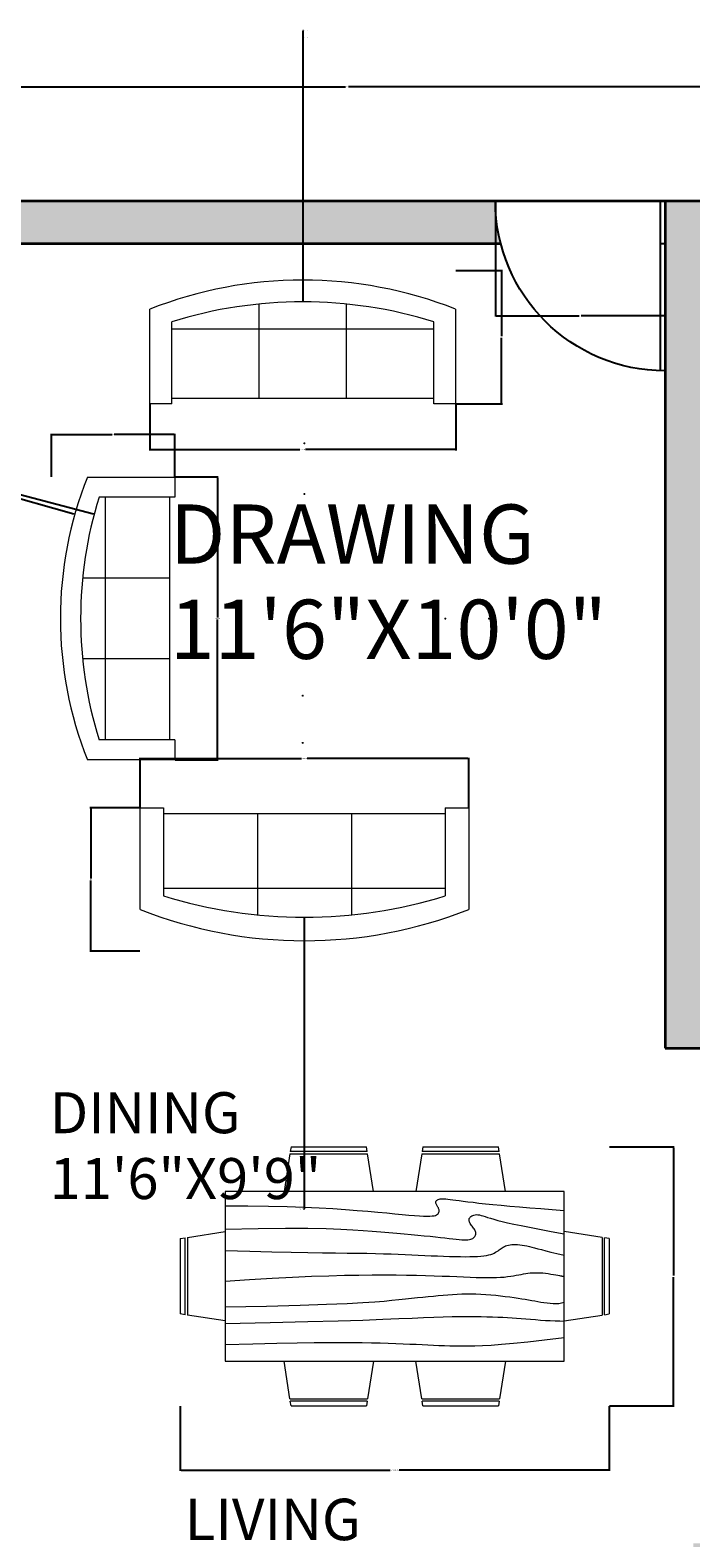
# Model space of a CAD drawing. Units: inches. Extents: x 582 to 1090, y 270 to 781.
# Tile 4 of 5: x 769 to 909, y 461 to 781. Entities that reach past the tile are written whole.
import ezdxf

# ---------------------------------------------------------------- set-up
doc = ezdxf.new("R2010")
doc.units = ezdxf.units.IN
doc.header["$MEASUREMENT"] = 0
for name, color, linetype, lineweight in [('A-ANNO-DIMS', 2, 'Continuous', 18), ('A-AREA-IDEN', 7, 'Continuous', 25), ('A-DOOR', 3, 'Continuous', 25), ('A-FURN', 8, 'Continuous', 18), ('A-WALL', 7, 'Continuous', 35)]:
    doc.layers.add(name, color=color, linetype=linetype, lineweight=lineweight)
doc.layers.add('A-WALL-PATT', color=9, linetype='Continuous', lineweight=13, true_color=0xc7c8ca)
doc.styles.get("Standard").update_dxf_attribs({"font": 'arial.ttf'})
doc.dimstyles.get("Standard").update_dxf_attribs({"dimtxt": 0.18, "dimasz": 0.18, "dimexe": 0.18, "dimexo": 0.0625, "dimgap": 0.09, "dimtad": 0, "dimtih": 1, "dimtoh": 1, "dimdec": 0, "dimzin": 0, "dimdsep": 46, "dimlunit": 3, "dimtxsty": 'Standard', "dimcen": 0.09, "dimadec": 0, "dimazin": 0, "dimtfac": 1, "dimtdec": 0, "dimtofl": 0, "dimtmove": 0, "dimatfit": 3, "dimfxl": 1, "dimtolj": 1, "dimtzin": 0, "dimarcsym": 0})

# ---------------------------------------------------------------- blocks, each defined once
blk = doc.blocks.new('Sofa - Roundback 7 ft.')
for p, q in [((-12.00002, -32.4421), (-12.00003, -6.5971)), ((11.99997, -32.4421), (11.99998, -6.5971)), ((-36.000027, -34), (-36.000027, -11.4696)), ((35.99998, -34), (35.99998, -11.4696)), ((-35.999844, -13.3819), (35.9998, -13.3819)), ((-36.000027, -32.4421), (35.99998, -32.4421))]:
    blk.add_line(p, q)
for points in [[(-36.000027, -34), (-42.000027, -34), (-42.000027, -8)], [(41.99998, -8), (41.99998, -34), (35.99998, -34)]]:
    blk.add_lwpolyline(points)
for centre, radius, start, end in [((0, -114.25), 114.25, 68.43141, 111.5686), ((-0.00001, -127.1968), 121.1968, 72.72033, 107.2797)]:
    blk.add_arc(centre, radius, start, end)
blk = doc.blocks.new('Dining Set - 36 x 72 in.')
for p, q in [((-22.2343, 26.00059), (-23.4847, 17.99762)), ((-22.2304, 26), (-5.7608, 26)), ((-22, 27.5), (-22.1562, 26.50042)), ((-5.8416, 26.5), (-22.1534, 26.5)), ((-22, 27.5), (-6, 27.5)), ((-5.8437, 26.49966), (-6, 27.5)), ((-4.5152, 17.99762), (-5.7655, 25.99926)), ((5.7657, 26.00059), (4.5153, 17.99762)), ((5.7696, 26), (22.2392, 26)), ((6, 27.5), (5.8438, 26.50042)), ((22.1584, 26.5), (5.8466, 26.5)), ((6, 27.5), (22, 27.5)), ((22.1563, 26.49966), (22, 27.5)), ((23.4848, 17.99762), (22.2345, 25.99926)), ((36, 18), (-36, 18)), ((-36, 18), (-36, -18)), ((36, -18), (36, 18)), ((-45.5, 8), (-44.5004, 8.15617)), ((-45.5, 8), (-45.5, -8)), ((-44.5, -8.15843), (-44.5, 8.15338)), ((-44.0006, 8.23428), (-35.9976, 9.48474)), ((-44, 8.23041), (-44, -8.23915)), ((44.0006, 8.23428), (35.9976, 9.48474)), ((44, 8.23041), (44, -8.23915)), ((44.5, -8.15843), (44.5, 8.15338)), ((45.5, 8), (44.5005, 8.15617)), ((45.5, 8), (45.5, -8)), ((-44.4997, -8.15631), (-45.5, -8)), ((-35.9976, -9.48476), (-43.9993, -8.2345)), ((35.9976, -9.48476), (43.9993, -8.2345)), ((44.4997, -8.15631), (45.5, -8)), ((-36, -18), (36, -18)), ((-22.2343, -26.0006), (-23.4847, -17.99762)), ((-4.5152, -17.99762), (-5.7655, -25.99928)), ((5.7657, -26.0006), (4.5153, -17.99762)), ((23.4848, -17.99762), (22.2345, -25.99928)), ((-22.2304, -26), (-5.7608, -26)), ((-22, -27.5), (-22.1562, -26.50044)), ((-5.8416, -26.5), (-22.1534, -26.5)), ((-22, -27.5), (-6, -27.5)), ((-5.8437, -26.49967), (-6, -27.5)), ((5.7696, -26), (22.2392, -26)), ((6, -27.5), (5.8438, -26.50044)), ((22.1584, -26.5), (5.8466, -26.5)), ((6, -27.5), (22, -27.5)), ((22.1563, -26.49967), (22, -27.5))]:
    blk.add_line(p, q)
for points in [[(-36, 15), (-31.1772, 14.97754), (-26.8079, 14.91406), (-22.8538, 14.81543), (-19.276, 14.6875), (-16.0362, 14.53613), (-13.0957, 14.36718), (-10.4159, 14.18652), (-7.9583, 14), (-5.6904, 13.81315), (-3.6035, 13.63021), (-1.6954, 13.45508), (0.0365, 13.29166), (1.5945, 13.14388), (2.9811, 13.01562), (4.1988, 12.9108), (5.25, 12.83333), (6.1393, 12.78613), (6.8802, 12.76823), (7.4883, 12.77767), (7.9792, 12.8125), (8.3685, 12.87077), (8.6719, 12.95052), (8.9049, 13.0498), (9.0833, 13.16666), (9.2205, 13.29899), (9.3216, 13.44401), (9.3895, 13.59879), (9.4271, 13.76041), (9.4373, 13.92594), (9.4232, 14.09245), (9.3875, 14.257), (9.3333, 14.41666), (9.2638, 14.56917), (9.1836, 14.71484), (9.0975, 14.85465), (9.0104, 14.98958), (8.9272, 15.1206), (8.8529, 15.2487), (8.7922, 15.37483), (8.75, 15.5), (8.7305, 15.62467), (8.7344, 15.74739), (8.7617, 15.86621), (8.8125, 15.97916), (8.8867, 16.08431), (8.9844, 16.17968), (9.1055, 16.26334), (9.25, 16.33333), (9.4189, 16.38802), (9.6172, 16.42708), (9.8506, 16.45052), (10.125, 16.45833), (10.4463, 16.45052), (10.8203, 16.42708), (11.2529, 16.38802), (11.75, 16.33333), (12.3184, 16.26318), (12.9694, 16.17838), (13.7151, 16.07991), (14.5677, 15.96875), (15.5395, 15.84586), (16.6426, 15.71224), (17.8893, 15.56884), (19.2917, 15.41666), (20.859, 15.25667), (22.5879, 15.08984), (24.4721, 14.91715), (26.5052, 14.73958), (28.6809, 14.5581), (30.9929, 14.3737), (33.4347, 14.18733), (36, 14)], [(-36, 10), (-28.9766, 10.14274), (-23.1725, 10.20442), (-18.4241, 10.19775), (-14.5677, 10.13541), (-11.4399, 10.03011), (-8.877, 9.89453), (-6.7154, 9.74137), (-4.7917, 9.58333), (-2.9698, 9.43082), (-1.2246, 9.28515), (0.4415, 9.14534), (2.026, 9.01041), (3.5266, 8.87939), (4.9408, 8.7513), (6.266, 8.62516), (7.5, 8.5), (8.6411, 8.37549), (9.6914, 8.2539), (10.6538, 8.13818), (11.5312, 8.03125), (12.3267, 7.93603), (13.043, 7.85547), (13.6831, 7.79248), (14.25, 7.75), (14.7471, 7.7303), (15.1797, 7.73307), (15.5537, 7.75732), (15.875, 7.80208), (16.1494, 7.86637), (16.3828, 7.94922), (16.5811, 8.04964), (16.75, 8.16666), (16.8944, 8.29915), (17.0143, 8.44531), (17.1089, 8.60319), (17.1771, 8.77083), (17.218, 8.94629), (17.2305, 9.1276), (17.2137, 9.31282), (17.1667, 9.5), (17.0895, 9.6875), (16.987, 9.875), (16.8649, 10.0625), (16.7292, 10.25), (16.5856, 10.4375), (16.4401, 10.625), (16.2985, 10.8125), (16.1667, 11), (16.05, 11.18733), (15.9518, 11.3737), (15.8752, 11.5581), (15.8229, 11.73958), (15.798, 11.91715), (15.8034, 12.08984), (15.842, 12.25667), (15.9167, 12.41666), (16.0295, 12.56836), (16.1784, 12.70833), (16.3605, 12.83268), (16.5729, 12.9375), (16.8127, 13.01888), (17.0768, 13.07291), (17.3625, 13.0957), (17.6667, 13.08333), (17.9894, 13.03312), (18.3418, 12.94726), (18.7382, 12.82918), (19.1927, 12.68229), (19.7195, 12.51001), (20.3327, 12.31575), (21.0465, 12.10294), (21.875, 11.875), (22.8357, 11.63354), (23.959, 11.37304), (25.2786, 11.08618), (26.8282, 10.76562), (28.6414, 10.40405), (30.752, 9.99414), (33.1936, 9.52856), (36, 9)], [(-36, 5.5), (-30.7157, 5.3348), (-26.069, 5.20963), (-21.9946, 5.11767), (-18.4271, 5.05208), (-15.3009, 5.00602), (-12.5508, 4.97265), (-10.1112, 4.94515), (-7.9167, 4.91666), (-5.909, 4.88167), (-4.0586, 4.83984), (-2.3429, 4.79215), (-0.7396, 4.73958), (0.7739, 4.6831), (2.22, 4.6237), (3.6213, 4.56233), (5, 4.5), (6.373, 4.43782), (7.7344, 4.3776), (9.0723, 4.32129), (10.375, 4.27083), (11.6309, 4.22819), (12.8281, 4.19531), (13.9551, 4.17415), (15, 4.16666), (15.954, 4.17448), (16.819, 4.19791), (17.6001, 4.23698), (18.3021, 4.29166), (18.9299, 4.36198), (19.4883, 4.44791), (19.9823, 4.54948), (20.4167, 4.66666), (20.7969, 4.79899), (21.1302, 4.94401), (21.4245, 5.09879), (21.6875, 5.26041), (21.9271, 5.42594), (22.1511, 5.59245), (22.3672, 5.757), (22.5834, 5.91666), (22.8065, 6.06868), (23.0404, 6.21093), (23.2879, 6.34147), (23.5521, 6.45833), (23.8358, 6.55957), (24.142, 6.64323), (24.4735, 6.70735), (24.8334, 6.75), (25.2235, 6.76969), (25.642, 6.76692), (26.0858, 6.74267), (26.5521, 6.69791), (27.0379, 6.63362), (27.5404, 6.55078), (28.0565, 6.45036), (28.5834, 6.33333), (29.1242, 6.19987), (29.7071, 6.04687), (30.3661, 5.87044), (31.1354, 5.66666), (32.0493, 5.43164), (33.142, 5.16146), (34.4475, 4.85221), (36, 4.5)], [(-36, -1), (-30.7915, -0.6591), (-26.0195, -0.38216), (-21.6519, -0.16284), (-17.6563, 0.00521), (-14.0005, 0.12833), (-10.6523, 0.21289), (-7.5796, 0.26522), (-4.75, 0.29166), (-2.134, 0.29793), (0.2878, 0.28711), (2.5317, 0.26163), (4.6146, 0.22396), (6.5529, 0.17651), (8.3633, 0.12174), (10.0623, 0.06209), (11.6667, 0), (13.1899, -0.06201), (14.6341, -0.1211), (15.9982, -0.17432), (17.2813, -0.21875), (18.4823, -0.25147), (19.6003, -0.26953), (20.6343, -0.27002), (21.5834, -0.25), (22.4481, -0.20768), (23.2357, -0.14584), (23.9549, -0.06836), (24.6146, 0.02083), (25.2235, 0.11784), (25.7904, 0.21875), (26.3241, 0.31966), (26.8334, 0.41666), (27.3265, 0.50618), (27.8099, 0.58593), (28.2894, 0.65397), (28.7709, 0.70833), (29.2601, 0.74707), (29.763, 0.76823), (30.2855, 0.76985), (30.8334, 0.75), (31.4088, 0.70784), (31.9994, 0.64713), (32.589, 0.57275), (33.1615, 0.48958), (33.7008, 0.4025), (34.1908, 0.3164), (34.6153, 0.23616), (34.9584, 0.16666), (35.2099, 0.11165), (35.3848, 0.07031), (35.504, 0.04069), (35.5886, 0.02083), (35.6594, 0.00879), (35.7377, 0.0026), (35.8442, 0.00032), (36, 0)], [(-36, -6.5), (-27.1843, -6.31267), (-20.084, -6.1263), (-14.469, -5.9419), (-10.1094, -5.76042), (-6.7752, -5.58285), (-4.2363, -5.41016), (-2.2629, -5.24333), (-0.625, -5.08334), (0.8708, -4.93099), (2.2715, -4.78646), (3.5872, -4.64974), (4.8281, -4.52084), (6.0046, -4.39974), (7.127, -4.28646), (8.2053, -4.18099), (9.25, -4.08334), (10.2705, -3.99382), (11.2734, -3.91407), (12.2647, -3.84603), (13.25, -3.79167), (14.2354, -3.75293), (15.2266, -3.73177), (16.2295, -3.73015), (17.25, -3.75), (18.2912, -3.79248), (19.3451, -3.85547), (20.4009, -3.93604), (21.4479, -4.03125), (22.4754, -4.13819), (23.4727, -4.25391), (24.4289, -4.37549), (25.3334, -4.5), (26.1785, -4.62492), (26.9694, -4.74935), (27.7145, -4.87281), (28.4219, -4.99479), (29.1, -5.11483), (29.7572, -5.23242), (30.4016, -5.34709), (31.0417, -5.45834), (31.6837, -5.56437), (32.3262, -5.65821), (32.9658, -5.73153), (33.599, -5.77604), (34.2224, -5.78345), (34.8327, -5.74545), (35.4264, -5.65373), (36, -5.5)], [(-36, -10), (-26.4022, -9.81299), (-18.4675, -9.62891), (-11.9839, -9.45069), (-6.7396, -9.28125), (-2.5226, -9.12354), (0.8789, -8.98047), (3.6769, -8.85498), (6.0833, -8.75), (8.2767, -8.66765), (10.3021, -8.60677), (12.1712, -8.56543), (13.8958, -8.54167), (15.4876, -8.53353), (16.9583, -8.53907), (18.3197, -8.55632), (19.5834, -8.58334), (20.7616, -8.61841), (21.8685, -8.66081), (22.9188, -8.71004), (23.9271, -8.76563), (24.9081, -8.82707), (25.8763, -8.89388), (26.8465, -8.96558), (27.8334, -9.04167), (28.8474, -9.12118), (29.8828, -9.20117), (30.93, -9.27824), (31.9792, -9.34896), (33.0205, -9.40991), (34.0443, -9.45768), (35.0407, -9.48885), (36, -9.5)], [(-36, -14.5), (-30.0881, -14.33513), (-25.0332, -14.21224), (-20.7312, -14.12647), (-17.0781, -14.07292), (-13.97, -14.04671), (-11.3027, -14.04297), (-8.9724, -14.05681), (-6.875, -14.08334), (-4.9224, -14.11833), (-3.0905, -14.16016), (-1.3709, -14.20785), (0.2448, -14.26042), (1.7647, -14.3169), (3.1973, -14.3763), (4.5507, -14.43767), (5.8333, -14.5), (7.0554, -14.5621), (8.235, -14.62175), (9.3922, -14.67652), (10.5469, -14.72396), (11.7192, -14.76164), (12.929, -14.78711), (14.1965, -14.79794), (15.5417, -14.79167), (16.9933, -14.76424), (18.6152, -14.70508), (20.4804, -14.60197), (22.6615, -14.44271), (25.2312, -14.21509), (28.2624, -13.9069), (31.8277, -13.50594), (36, -13)]]:
    blk.add_lwpolyline(points)
blk = doc.blocks.new('DOOR-SINGLE-36IN')
for p, q in [((35, 0), (35, 36)), ((36, 0), (36, 36))]:
    blk.add_line(p, q)
blk.add_arc((36, 0), 36, 90, 180)
blk = doc.blocks.new('*D16')
at = {"layer": 'A-ANNO-DIMS', "color": 0, "lineweight": -2, "transparency": 16777216}
for p, q in [((794.48, 701.38), (794.48, 691.53)), ((859.38, 701.38), (859.38, 691.53)), ((794.66, 691.71), (826.33, 691.71)), ((859.2, 691.71), (827.53, 691.71))]:
    blk.add_line(p, q, dxfattribs=at)
at = {"layer": 'A-ANNO-DIMS', "color": 0, "transparency": 16777216}
for points in [[(794.66, 691.74), (794.66, 691.68), (794.48, 691.71)], [(859.2, 691.74), (859.2, 691.68), (859.38, 691.71)]]:
    blk.add_solid(points, dxfattribs=at)
at = {"layer": 'Defpoints', "color": 0, "transparency": 16777216}
for p in [(794.48, 701.45), (859.38, 701.45), (859.38, 691.71)]:
    blk.add_point(p, dxfattribs=at)
at = {"layer": 'A-ANNO-DIMS', "color": 0, "transparency": 16777216, "insert": (826.93, 691.71), "char_height": 0.18, "attachment_point": 5}
blk.add_mtext('\\A1;SOFA 65', dxfattribs=at)
blk = doc.blocks.new('*D17')
at = {"layer": 'A-ANNO-DIMS', "color": 0, "lineweight": -2, "transparency": 16777216}
for p, q in [((859.44, 729.77), (869.29, 729.77)), ((869.11, 729.59), (869.11, 715.79)), ((869.11, 701.63), (869.11, 715.43)), ((859.44, 701.45), (869.29, 701.45))]:
    blk.add_line(p, q, dxfattribs=at)
at = {"layer": 'A-ANNO-DIMS', "color": 0, "transparency": 16777216}
for points in [[(869.08, 729.59), (869.14, 729.59), (869.11, 729.77)], [(869.08, 701.63), (869.14, 701.63), (869.11, 701.45)]]:
    blk.add_solid(points, dxfattribs=at)
at = {"layer": 'Defpoints', "color": 0, "transparency": 16777216}
for p in [(859.38, 729.77), (869.11, 729.77), (859.38, 701.45)]:
    blk.add_point(p, dxfattribs=at)
at = {"layer": 'A-ANNO-DIMS', "color": 0, "transparency": 16777216, "insert": (869.11, 715.61), "char_height": 0.18, "attachment_point": 5}
blk.add_mtext('\\A1;28', dxfattribs=at)
blk = doc.blocks.new('*D18')
at = {"layer": 'A-ANNO-DIMS', "color": 0, "lineweight": -2, "transparency": 16777216}
for p, q in [((799.87, 685.89), (809, 685.89)), ((808.82, 685.71), (808.82, 656.03)), ((808.82, 625.98), (808.82, 655.66)), ((799.87, 625.8), (809, 625.8))]:
    blk.add_line(p, q, dxfattribs=at)
at = {"layer": 'A-ANNO-DIMS', "color": 0, "transparency": 16777216}
for points in [[(808.79, 685.71), (808.85, 685.71), (808.82, 685.89)], [(808.79, 625.98), (808.85, 625.98), (808.82, 625.8)]]:
    blk.add_solid(points, dxfattribs=at)
at = {"layer": 'Defpoints', "color": 0, "transparency": 16777216}
for p in [(799.8, 685.89), (808.82, 685.89), (799.8, 625.8)]:
    blk.add_point(p, dxfattribs=at)
at = {"layer": 'A-ANNO-DIMS', "color": 0, "transparency": 16777216, "insert": (808.82, 655.84), "char_height": 0.18, "attachment_point": 5}
blk.add_mtext('\\A1;SOFA 60', dxfattribs=at)
blk = doc.blocks.new('*D19')
at = {"layer": 'A-ANNO-DIMS', "color": 0, "lineweight": -2, "transparency": 16777216}
for p, q in [((773.58, 685.95), (773.58, 695.08)), ((773.76, 694.9), (786.47, 694.9)), ((799.62, 694.9), (786.91, 694.9)), ((799.8, 685.95), (799.8, 695.08))]:
    blk.add_line(p, q, dxfattribs=at)
at = {"layer": 'A-ANNO-DIMS', "color": 0, "transparency": 16777216}
for points in [[(773.76, 694.93), (773.76, 694.87), (773.58, 694.9)], [(799.62, 694.93), (799.62, 694.87), (799.8, 694.9)]]:
    blk.add_solid(points, dxfattribs=at)
at = {"layer": 'Defpoints', "color": 0, "transparency": 16777216}
for p in [(773.58, 694.9), (773.58, 685.89), (799.8, 685.89)]:
    blk.add_point(p, dxfattribs=at)
at = {"layer": 'A-ANNO-DIMS', "color": 0, "transparency": 16777216, "insert": (786.69, 694.9), "char_height": 0.18, "attachment_point": 5}
blk.add_mtext('\\A1;26', dxfattribs=at)
blk = doc.blocks.new('*D20')
at = {"layer": 'A-ANNO-DIMS', "color": 0, "lineweight": -2, "transparency": 16777216}
for p, q in [((792.4, 615.7), (792.4, 626.28)), ((792.58, 626.1), (826.68, 626.1)), ((861.98, 626.1), (827.87, 626.1)), ((862.16, 615.7), (862.16, 626.28))]:
    blk.add_line(p, q, dxfattribs=at)
at = {"layer": 'A-ANNO-DIMS', "color": 0, "transparency": 16777216}
for points in [[(792.58, 626.13), (792.58, 626.07), (792.4, 626.1)], [(861.98, 626.13), (861.98, 626.07), (862.16, 626.1)]]:
    blk.add_solid(points, dxfattribs=at)
at = {"layer": 'Defpoints', "color": 0, "transparency": 16777216}
for p in [(792.4, 626.1), (792.4, 615.64), (862.16, 615.64)]:
    blk.add_point(p, dxfattribs=at)
at = {"layer": 'A-ANNO-DIMS', "color": 0, "transparency": 16777216, "insert": (827.28, 626.1), "char_height": 0.18, "attachment_point": 5}
blk.add_mtext('\\A1;SOFA 70', dxfattribs=at)
blk = doc.blocks.new('*D21')
at = {"layer": 'A-ANNO-DIMS', "color": 0, "lineweight": -2, "transparency": 16777216}
for p, q in [((792.33, 615.64), (781.75, 615.64)), ((781.93, 615.46), (781.93, 600.59)), ((781.93, 585.37), (781.93, 600.23)), ((792.33, 585.19), (781.75, 585.19))]:
    blk.add_line(p, q, dxfattribs=at)
at = {"layer": 'A-ANNO-DIMS', "color": 0, "transparency": 16777216}
for points in [[(781.9, 615.46), (781.96, 615.46), (781.93, 615.64)], [(781.9, 585.37), (781.96, 585.37), (781.93, 585.19)]]:
    blk.add_solid(points, dxfattribs=at)
at = {"layer": 'Defpoints', "color": 0, "transparency": 16777216}
for p in [(792.4, 615.64), (781.93, 585.19), (792.4, 585.19)]:
    blk.add_point(p, dxfattribs=at)
at = {"layer": 'A-ANNO-DIMS', "color": 0, "transparency": 16777216, "insert": (781.93, 600.41), "char_height": 0.18, "attachment_point": 5}
blk.add_mtext('\\A1;30', dxfattribs=at)
blk = doc.blocks.new('*D30')
at = {"layer": 'A-ANNO-DIMS', "color": 0, "lineweight": -2, "transparency": 16777216}
for p, q in [((800.94, 488.57), (800.94, 474.8)), ((891.94, 488.57), (891.94, 474.8)), ((801.12, 474.98), (845.48, 474.98)), ((891.76, 474.98), (847.39, 474.98))]:
    blk.add_line(p, q, dxfattribs=at)
at = {"layer": 'A-ANNO-DIMS', "color": 0, "transparency": 16777216}
for points in [[(801.12, 475.01), (801.12, 474.95), (800.94, 474.98)], [(891.76, 475.01), (891.76, 474.95), (891.94, 474.98)]]:
    blk.add_solid(points, dxfattribs=at)
at = {"layer": 'Defpoints', "color": 0, "transparency": 16777216}
for p in [(800.94, 488.63), (891.94, 488.63), (891.94, 474.98)]:
    blk.add_point(p, dxfattribs=at)
at = {"layer": 'A-ANNO-DIMS', "color": 0, "transparency": 16777216, "insert": (846.44, 474.98), "char_height": 0.18, "attachment_point": 5}
blk.add_mtext('\\A1;DINING SET 91', dxfattribs=at)
blk = doc.blocks.new('*D31')
at = {"layer": 'A-ANNO-DIMS', "color": 0, "lineweight": -2, "transparency": 16777216}
for p, q in [((892, 543.63), (905.77, 543.63)), ((905.59, 543.45), (905.59, 516.32)), ((905.59, 488.81), (905.59, 515.95)), ((892, 488.63), (905.77, 488.63))]:
    blk.add_line(p, q, dxfattribs=at)
at = {"layer": 'A-ANNO-DIMS', "color": 0, "transparency": 16777216}
for points in [[(905.56, 543.45), (905.62, 543.45), (905.59, 543.63)], [(905.56, 488.81), (905.62, 488.81), (905.59, 488.63)]]:
    blk.add_solid(points, dxfattribs=at)
at = {"layer": 'Defpoints', "color": 0, "transparency": 16777216}
for p in [(891.94, 543.63), (905.59, 543.63), (891.94, 488.63)]:
    blk.add_point(p, dxfattribs=at)
at = {"layer": 'A-ANNO-DIMS', "color": 0, "transparency": 16777216, "insert": (905.59, 516.13), "char_height": 0.18, "attachment_point": 5}
blk.add_mtext('\\A1;55', dxfattribs=at)
blk = doc.blocks.new('*D34')
at = {"layer": 'A-ANNO-DIMS', "color": 0, "lineweight": -2, "transparency": 16777216}
for p, q in [((606.8, 744.51), (606.8, 768.93)), ((606.98, 768.75), (836.01, 768.75)), ((1065.62, 768.75), (836.6, 768.75)), ((1065.8, 744.51), (1065.8, 768.93))]:
    blk.add_line(p, q, dxfattribs=at)
at = {"layer": 'A-ANNO-DIMS', "color": 0, "transparency": 16777216}
for points in [[(606.98, 768.78), (606.98, 768.72), (606.8, 768.75)], [(1065.62, 768.78), (1065.62, 768.72), (1065.8, 768.75)]]:
    blk.add_solid(points, dxfattribs=at)
at = {"layer": 'Defpoints', "color": 0, "transparency": 16777216}
for p in [(1065.8, 768.75), (606.8, 744.45), (1065.8, 744.45)]:
    blk.add_point(p, dxfattribs=at)
at = {"layer": 'A-ANNO-DIMS', "color": 0, "transparency": 16777216, "insert": (836.3, 768.75), "char_height": 0.18, "attachment_point": 5}
blk.add_mtext('\\A1;459', dxfattribs=at)
blk = doc.blocks.new('*D35')
at = {"layer": 'A-ANNO-DIMS', "color": 0, "lineweight": -2, "transparency": 16777216}
for p, q in [((867.8, 744.38), (867.8, 719.97)), ((903.8, 744.38), (903.8, 719.97)), ((867.98, 720.15), (885.59, 720.15)), ((903.62, 720.15), (886.02, 720.15))]:
    blk.add_line(p, q, dxfattribs=at)
at = {"layer": 'A-ANNO-DIMS', "color": 0, "transparency": 16777216}
for points in [[(867.98, 720.18), (867.98, 720.12), (867.8, 720.15)], [(903.62, 720.18), (903.62, 720.12), (903.8, 720.15)]]:
    blk.add_solid(points, dxfattribs=at)
at = {"layer": 'Defpoints', "color": 0, "transparency": 16777216}
for p in [(867.8, 744.45), (903.8, 744.45), (867.8, 720.15)]:
    blk.add_point(p, dxfattribs=at)
at = {"layer": 'A-ANNO-DIMS', "color": 0, "transparency": 16777216, "insert": (885.8, 720.15), "char_height": 0.18, "attachment_point": 5}
blk.add_mtext('\\A1;36', dxfattribs=at)
blk = doc.blocks.new('*D69')
at = {"layer": 'A-ANNO-DIMS', "color": 0, "lineweight": -2, "transparency": 16777216}
for p, q in [((827.19, 693.04), (827.37, 693.04)), ((827.28, 692.95), (827.28, 693.13)), ((827.28, 531.99), (827.28, 592.2)), ((827.1, 531.99), (827.28, 531.99))]:
    blk.add_line(p, q, dxfattribs=at)
at = {"layer": 'A-ANNO-DIMS', "color": 0, "transparency": 16777216}
blk.add_solid([(827.25, 592.2), (827.31, 592.2), (827.28, 592.38)], dxfattribs=at)
at = {"layer": 'Defpoints', "color": 0, "transparency": 16777216}
for p in [(827.28, 693.04), (827.28, 592.38)]:
    blk.add_point(p, dxfattribs=at)
at = {"layer": 'A-ANNO-DIMS', "color": 0, "transparency": 16777216, "insert": (826.55, 531.99), "char_height": 0.18, "attachment_point": 5}
blk.add_mtext('\\A1;R100.65', dxfattribs=at)
blk = doc.blocks.new('*D71')
at = {"layer": 'A-ANNO-DIMS', "color": 0, "lineweight": -2, "transparency": 16777216}
for p, q in [((827.19, 682.29), (827.37, 682.29)), ((827.28, 682.2), (827.28, 682.38)), ((827.28, 530.47), (827.28, 587.22)), ((827.1, 530.47), (827.28, 530.47))]:
    blk.add_line(p, q, dxfattribs=at)
at = {"layer": 'A-ANNO-DIMS', "color": 0, "transparency": 16777216}
blk.add_solid([(827.25, 587.22), (827.31, 587.22), (827.28, 587.4)], dxfattribs=at)
at = {"layer": 'Defpoints', "color": 0, "transparency": 16777216}
for p in [(827.28, 682.29), (827.28, 587.4)]:
    blk.add_point(p, dxfattribs=at)
at = {"layer": 'A-ANNO-DIMS', "color": 0, "transparency": 16777216, "insert": (826.62, 530.47), "char_height": 0.18, "attachment_point": 5}
blk.add_mtext('\\A1;R94.88', dxfattribs=at)
blk = doc.blocks.new('*D72')
at = {"layer": 'A-ANNO-DIMS', "color": 0, "lineweight": -2, "transparency": 16777216}
for p, q in [((827.11, 779.25), (826.93, 779.25)), ((826.93, 779.25), (826.93, 723.26)), ((826.84, 629.45), (827.02, 629.45)), ((826.93, 629.36), (826.93, 629.54))]:
    blk.add_line(p, q, dxfattribs=at)
at = {"layer": 'A-ANNO-DIMS', "color": 0, "transparency": 16777216}
blk.add_solid([(826.9, 723.26), (826.96, 723.26), (826.93, 723.08)], dxfattribs=at)
at = {"layer": 'Defpoints', "color": 0, "transparency": 16777216}
for p in [(826.93, 723.08), (826.93, 629.45)]:
    blk.add_point(p, dxfattribs=at)
at = {"layer": 'A-ANNO-DIMS', "color": 0, "transparency": 16777216, "insert": (827.59, 779.25), "char_height": 0.18, "attachment_point": 5}
blk.add_mtext('\\A1;R93.63', dxfattribs=at)
blk = doc.blocks.new('*D74')
at = {"layer": 'A-ANNO-DIMS', "color": 0, "lineweight": -2, "transparency": 16777216}
for p, q in [((827.11, 780.67), (826.93, 780.67)), ((826.93, 780.67), (826.93, 727.89)), ((826.84, 639.45), (827.02, 639.45)), ((826.93, 639.36), (826.93, 639.54))]:
    blk.add_line(p, q, dxfattribs=at)
at = {"layer": 'A-ANNO-DIMS', "color": 0, "transparency": 16777216}
blk.add_solid([(826.9, 727.89), (826.96, 727.89), (826.93, 727.71)], dxfattribs=at)
at = {"layer": 'Defpoints', "color": 0, "transparency": 16777216}
for p in [(826.93, 727.71), (826.93, 639.45)]:
    blk.add_point(p, dxfattribs=at)
at = {"layer": 'A-ANNO-DIMS', "color": 0, "transparency": 16777216, "insert": (827.59, 780.67), "char_height": 0.18, "attachment_point": 5}
blk.add_mtext('\\A1;R88.26', dxfattribs=at)
blk = doc.blocks.new('*D75')
at = {"layer": 'A-ANNO-DIMS', "color": 0, "lineweight": -2, "transparency": 16777216}
for p, q in [((732.37, 691.29), (782.48, 678.04)), ((866.37, 655.84), (866.55, 655.84)), ((866.46, 655.75), (866.46, 655.93))]:
    blk.add_line(p, q, dxfattribs=at)
at = {"layer": 'A-ANNO-DIMS', "color": 0, "transparency": 16777216}
blk.add_solid([(782.49, 678.07), (782.47, 678.01), (782.66, 678)], dxfattribs=at)
at = {"layer": 'Defpoints', "color": 0, "transparency": 16777216}
for p in [(782.66, 678), (866.46, 655.84)]:
    blk.add_point(p, dxfattribs=at)
at = {"layer": 'A-ANNO-DIMS', "color": 0, "transparency": 16777216, "insert": (731.89, 691.29), "char_height": 0.18, "attachment_point": 5}
blk.add_mtext('\\A1;R86.69', dxfattribs=at)
blk = doc.blocks.new('*D76')
at = {"layer": 'A-ANNO-DIMS', "color": 0, "lineweight": -2, "transparency": 16777216}
for p, q in [((731.17, 691.3), (731.35, 691.3)), ((731.35, 691.3), (778.37, 678.05)), ((857.11, 655.84), (857.29, 655.84)), ((857.2, 655.75), (857.2, 655.93))]:
    blk.add_line(p, q, dxfattribs=at)
at = {"layer": 'A-ANNO-DIMS', "color": 0, "transparency": 16777216}
blk.add_solid([(778.38, 678.08), (778.37, 678.02), (778.55, 678)], dxfattribs=at)
at = {"layer": 'Defpoints', "color": 0, "transparency": 16777216}
for p in [(778.55, 678), (857.2, 655.84)]:
    blk.add_point(p, dxfattribs=at)
at = {"layer": 'A-ANNO-DIMS', "color": 0, "transparency": 16777216, "insert": (730.7, 691.3), "char_height": 0.18, "attachment_point": 5}
blk.add_mtext('\\A1;R81.72', dxfattribs=at)

msp = doc.modelspace()

# ---------------------------------------------------------------- hatches: boundary and pattern name
at = {"layer": 'A-WALL-PATT'}
h = msp.add_hatch(color=256, dxfattribs=at)
h.dxf.hatch_style = 1
h.paths.add_polyline_path([(867.8047, 744.446), (765.8047, 744.446), (606.8047, 744.446), (606.8047, 711.9379), (615.8047, 711.9379), (615.8047, 735.446), (756.8047, 735.446), (756.8047, 585.446), (765.8047, 585.446), (765.8047, 735.446), (868.9478, 735.446, -0.06325422)])
h.paths.add_polyline_path([(1065.8047, 744.446), (912.8047, 744.446), (903.8047, 744.446), (903.8047, 708.446), (903.8047, 594.446), (903.8047, 564.6071), (912.8047, 564.6071), (912.8047, 600.6071), (912.8047, 735.446), (1056.8047, 735.446), (1056.8047, 720.2375), (1065.8047, 720.2375)])
h.paths.add_polyline_path([(1065.8047, 632.4383), (1056.8047, 632.4383), (1056.8047, 594.446), (1056.8047, 584.9343), (1065.8047, 584.9343), (1065.8047, 594.446)], flags=17)
h.paths.add_polyline_path([(1056.8047, 603.446), (951.8047, 603.446), (951.8047, 594.446), (1056.8047, 594.446)], flags=17)
h.paths.add_polyline_path([(1065.8047, 525.446), (1065.8047, 550.2593), (1056.8047, 550.2593), (1056.8047, 534.446), (960.8047, 534.446), (960.8047, 565.946, -0.07397332), (952.1262, 564.6071), (951.8047, 564.6071), (951.8047, 495.446, -0.07632083), (960.8047, 494.0641), (960.8047, 525.446), (1056.8047, 525.446), (1056.8047, 508.8565), (1065.8047, 508.8565)])
h.paths.add_polyline_path([(1065.8047, 478.2143), (1056.8047, 478.2143), (1056.8047, 465.446), (951.8047, 465.446), (951.8047, 456.446), (1056.8047, 456.446), (1056.8047, 420.446), (1065.8047, 420.446), (1065.8047, 456.446)])
h.paths.add_polyline_path([(1065.8047, 420.446), (1056.8047, 420.446), (1017.8047, 420.446), (1017.8047, 456.446), (1008.8047, 456.446), (1008.8047, 411.446), (1038.8047, 411.446), (1065.8047, 411.446)])
h.paths.add_polyline_path([(1065.8047, 411.446), (1056.8047, 411.446), (1056.8047, 327.446), (1065.8047, 327.446)])
h.paths.add_polyline_path([(1065.8047, 327.446), (1056.8047, 327.446), (1017.8047, 327.446), (1017.8047, 382.8278, -0.07632083), (1008.8047, 381.446), (1008.8047, 327.446), (983.7348, 327.446), (983.7348, 318.446), (1065.8047, 318.446)])
h.paths.add_polyline_path([(946.9624, 327.446), (918.8047, 327.446), (918.8047, 369.8742), (918.8047, 459.446), (909.8047, 459.446), (909.8047, 369.8742), (909.8047, 318.446), (946.9624, 318.446)])
h.paths.add_polyline_path([(918.8047, 318.446), (909.8047, 318.446), (909.8047, 303.4372), (765.8047, 303.4372), (765.8047, 327.446), (756.8047, 327.446), (756.8047, 294.4372), (918.8047, 294.4372)])
h.paths.add_polyline_path([(909.8047, 378.8742), (882.3477, 378.8742), (882.3477, 347.0959), (889.3299, 347.0959), (889.3299, 369.8742), (909.8047, 369.8742)])
h.paths.add_polyline_path([(779.4225, 378.8742), (765.8047, 378.8742), (765.8047, 369.8742), (779.4225, 369.8742)])
h.paths.add_polyline_path([(765.8047, 516.446), (756.8047, 516.446), (756.8047, 480.446), (756.8047, 336.446), (724.1731, 336.446), (724.1731, 327.446), (765.8047, 327.446), (765.8047, 369.8742), (765.8047, 378.8742)])
h.paths.add_polyline_path([(615.8047, 516.446), (606.8047, 516.446), (606.8047, 327.446), (637.062, 327.446), (637.062, 336.446), (615.8047, 336.446)])
h.paths.add_polyline_path([(615.8047, 631.6498), (606.8047, 631.6498), (606.8047, 585.446), (606.8047, 569.338), (615.8047, 569.338), (615.8047, 585.446), (615.8047, 594.446)])
h.paths.add_polyline_path([(721.9478, 594.446), (615.8047, 594.446), (615.8047, 585.446), (627.9505, 585.446, -0.03261849), (629.8936, 585.446), (710.8047, 585.446), (710.8047, 525.446), (675.3033, 525.446), (675.3033, 516.446), (719.8047, 516.446), (720.8047, 516.446), (720.8047, 525.446), (719.8047, 525.446), (719.8047, 585.446), (720.8047, 585.446, -0.06325422)])
h.paths.add_polyline_path([(646.6852, 525.446), (615.8047, 525.446), (615.8047, 516.446), (645.3033, 516.446, -0.07632083)])
h.paths.add_polyline_path([(615.8047, 525.446), (615.8047, 539.7667), (606.8047, 539.7667), (606.8047, 516.446), (615.8047, 516.446)])

# ---------------------------------------------------------------- linework, layer by layer
at = {"layer": 'A-DOOR'}
for p, q in [((903.8047, 744.446), (867.8047, 744.446)), ((902.8047, 735.446), (903.8047, 735.446))]:
    msp.add_line(p, q, dxfattribs=at)
at = {"layer": 'A-WALL'}
for p, q in [((912.8047, 744.446), (765.8047, 744.446)), ((903.8047, 744.446), (903.8047, 594.446)), ((765.8047, 735.446), (868.9478, 735.446)), ((903.8047, 594.446), (903.8047, 564.6071)), ((903.8047, 564.6071), (912.8047, 564.6071))]:
    msp.add_line(p, q, dxfattribs=at)

# ---------------------------------------------------------------- block references
at = {"layer": 'A-DOOR', "extrusion": (0, 0, -1), "zscale": -1, "rotation": 180}
msp.add_blockref('DOOR-SINGLE-36IN', (-867.805, 744.4459), dxfattribs=at)
at = {"layer": 'A-FURN', "xscale": 0.7725365648415388, "yscale": 0.7725365648415388, "zscale": 0.7725365648415388}
msp.add_blockref('Sofa - Roundback 7 ft.', (826.9297, 727.7122), dxfattribs=at)
at = {"layer": 'A-FURN'}
for p, xscale, yscale, zscale, rotation in [((775.4862, 655.8447), 0.71524828031232, 0.71524828031232, 0.71524828031232, 90), ((827.277, 587.401), 0.8304959249008952, 0.8304959249008952, 0.8304959249008952, 180)]:
    msp.add_blockref('Sofa - Roundback 7 ft.', p, dxfattribs=dict(at, xscale=xscale, yscale=yscale, zscale=zscale, rotation=rotation))
msp.add_blockref('Dining Set - 36 x 72 in.', (846.4352, 516.134), dxfattribs=at)

# ---------------------------------------------------------------- texts
at = {"layer": 'A-ANNO-DIMS'}
for s, height, p in [('11\'6"X10\'0"', 12.580749, (798.6904, 647.2617)), ('11\'6"X9\'9"', 8.70803, (773.2222, 532.5374))]:
    msp.add_text(s, height=height, dxfattribs=at).set_placement(p)
at = {"layer": 'A-AREA-IDEN'}
for s, height, p in [('DRAWING ', 12.58075, (798.6904, 667.4716)), ('DINING', 8.70803, (773.2222, 546.5261)), ('LIVING', 8.79628, (801.8638, 460.1026))]:
    msp.add_text(s, height=height, dxfattribs=at).set_placement(p)

# ---------------------------------------------------------------- dimensions: what is measured, and where the dimension line sits
at = {"layer": 'A-ANNO-DIMS'}
for center, mpoint, picture, middle in [((826.9297, 639.4499), (826.93, 727.7122), '*D74', (827.5899, 780.6696)), ((826.9297, 629.448), (826.93, 723.077), '*D72', (827.59, 779.2544)), ((827.277, 693.0374), (827.277, 592.384), '*D69', (826.5466, 531.9919)), ((857.2034, 655.8447), (778.5479, 678.0034), '*D76', (730.6957, 691.2986)), ((866.4635, 655.8447), (782.6557, 677.9959), '*D75', (732.371, 691.2866)), ((827.277, 682.2852), (827.277, 587.401), '*D71', (826.617, 530.4705))]:
    dim = msp.add_radius_dim(center=center, mpoint=mpoint, dimstyle='Standard', override={"dimdec": 2, "dimlfac": 1, "dimrnd": 0, "dimzin": 0, "dimdsep": 46, "dimlunit": 2}, dxfattribs=at)
    dim.commit()
    dim.dimension.update_dxf_attribs({"geometry": picture, "text_midpoint": middle, "dimtype": 164})
dim = msp.add_linear_dim(base=(1065.8047, 768.746), p1=(606.8047, 744.446), p2=(1065.8047, 744.446), dimstyle='Standard', override={"dimdec": 0, "dimlfac": 1, "dimrnd": 0, "dimzin": 0, "dimdsep": 46, "dimlunit": 2}, dxfattribs=at)
dim.commit()
dim.dimension.update_dxf_attribs({"geometry": '*D34', "text_midpoint": (836.3047, 768.746)})
for base, p1, p2, angle, picture, middle in [((867.8047, 720.146), (903.8047, 744.446), (867.8047, 744.446), 180, '*D35', (885.8047, 720.146)), ((869.1102, 729.7723), (859.3762, 701.446), (859.3762, 729.7723), 90, '*D17', (869.1102, 715.6091)), ((773.5789, 694.8972), (799.8047, 685.8851), (773.5789, 685.8851), 180, '*D19', (786.6918, 694.8972)), ((781.9319, 585.1863), (792.3962, 615.6379), (792.3962, 585.1863), 270, '*D21', (781.9319, 600.4121)), ((905.5852, 543.634), (891.9352, 488.634), (891.9352, 543.634), 90, '*D31', (905.5852, 516.134))]:
    dim = msp.add_linear_dim(base=base, p1=p1, p2=p2, angle=angle, dimstyle='Standard', override={"dimdec": 0, "dimlfac": 1, "dimrnd": 0, "dimzin": 0, "dimdsep": 46, "dimlunit": 2}, dxfattribs=at)
    dim.commit()
    dim.dimension.update_dxf_attribs({"geometry": picture, "text_midpoint": middle})
for base, p1, p2, text, picture, middle in [((859.3762, 691.712), (794.4832, 701.446), (859.3762, 701.446), 'SOFA <>', '*D16', (826.9297, 691.712)), ((891.9352, 474.984), (800.9352, 488.634), (891.9352, 488.634), 'DINING SET <>', '*D30', (846.4352, 474.984))]:
    dim = msp.add_linear_dim(base=base, p1=p1, p2=p2, text=text, dimstyle='Standard', override={"dimdec": 0, "dimlfac": 1, "dimrnd": 0, "dimzin": 0, "dimdsep": 46, "dimlunit": 2}, dxfattribs=at)
    dim.commit()
    dim.dimension.update_dxf_attribs({"geometry": picture, "text_midpoint": middle})
for base, p1, p2, angle, picture, middle in [((808.8168, 685.8851), (799.8047, 625.8042), (799.8047, 685.8851), 90, '*D18', (808.8168, 655.8447)), ((792.3962, 626.1021), (862.1578, 615.6379), (792.3962, 615.6379), 180, '*D20', (827.277, 626.1021))]:
    dim = msp.add_linear_dim(base=base, p1=p1, p2=p2, angle=angle, text='SOFA <>', dimstyle='Standard', override={"dimdec": 0, "dimlfac": 1, "dimrnd": 0, "dimzin": 0, "dimdsep": 46, "dimlunit": 2}, dxfattribs=at)
    dim.commit()
    dim.dimension.update_dxf_attribs({"geometry": picture, "text_midpoint": middle})

doc.saveas('drawing.dxf')
